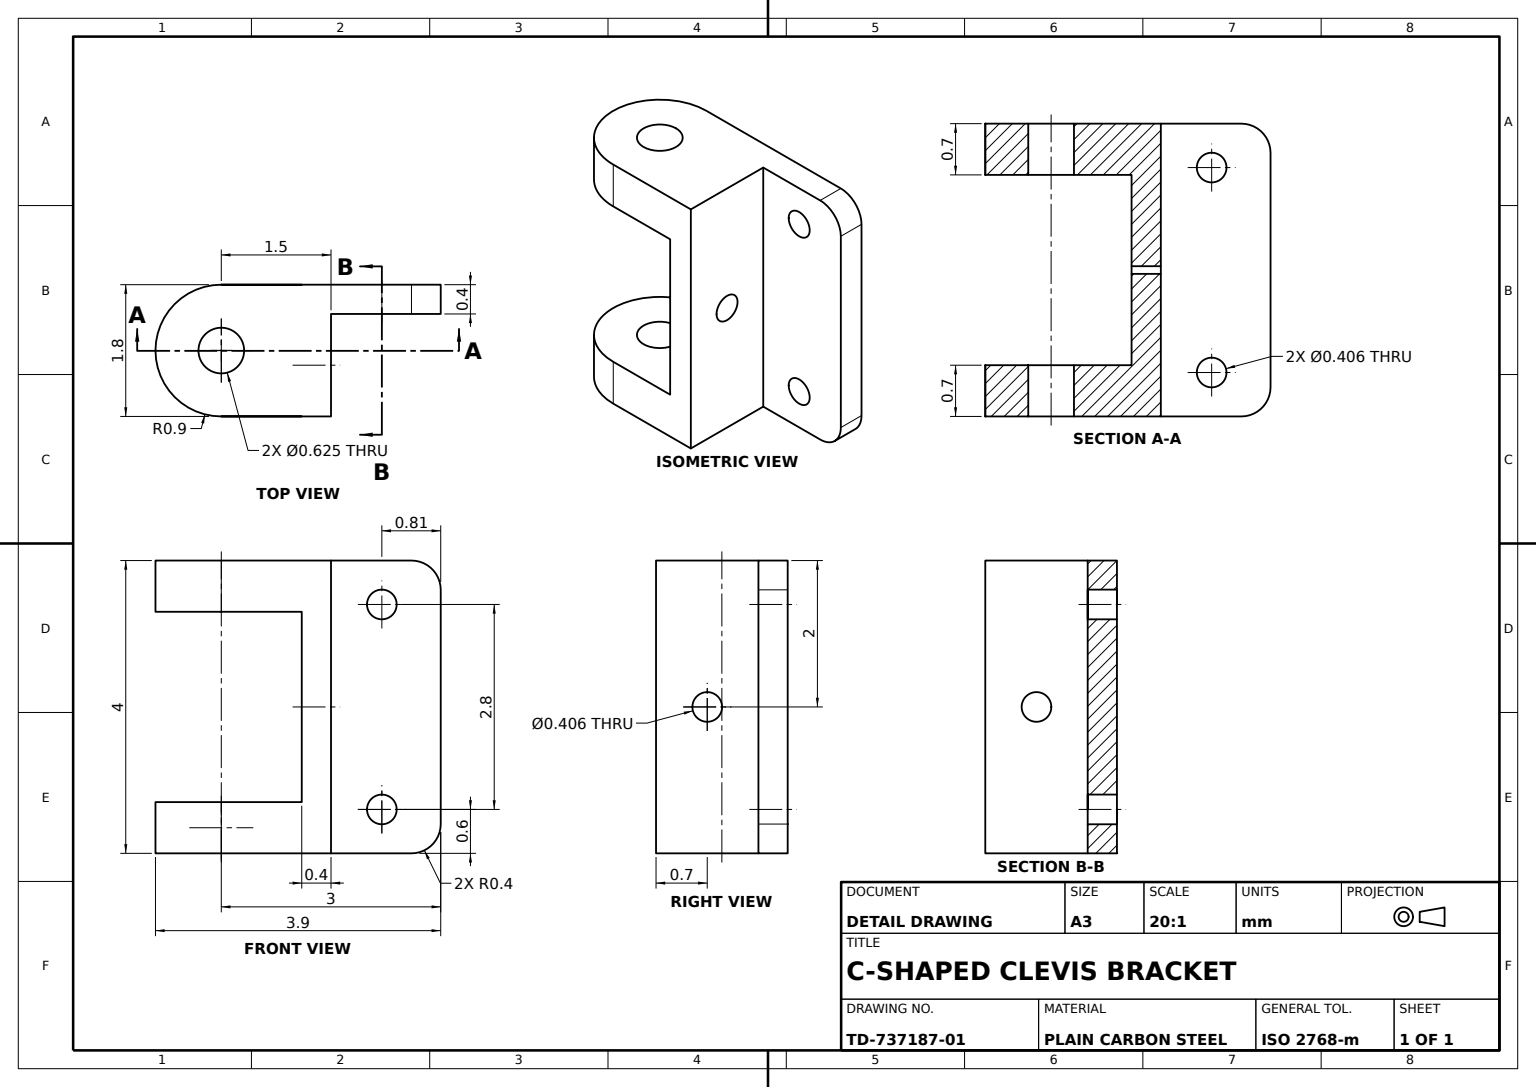
SolidWorks part; units mm, degrees
material "Plain Carbon Steel"
ref_plane "Front Plane" through (0, 0, 0) normal (0, 0, 1) x (1, 0, 0)
ref_plane "Top Plane" through (0, 0, 0) normal (0, 1, 0) x (1, 0, 0)
ref_plane "Right Plane" through (0, 0, 0) normal (1, 0, 0) x (0, 0, -1)
sketch "C-Frame Profile Sketch" plane through (0, 0, 0) normal (0, 0, 1) x (1, 0, 0)
  line L4 (0, 0) -> (2.6, 0)
  line L5 (2.6, -4) -> (0, -4)
  line L6 (0, -4) -> (0, 0)
  line L7 (0, 0) -> (3, 0)
  line L8 (3, -0.4) -> (3, -3.6)
  arc A0 (3, -0.4) -> (2.6, 0) centre (2.6, -0.4) ccw
  arc A1 (3, -3.6) -> (2.6, -4) centre (2.6, -3.6) cw
  point P11 (3, -4)
  dimension "D3" = 0.4
  dimension "D4" = 0.4
  dimension "D1" = 4
  dimension "D2" = 3
extrude "C-Frame Base" add sketch "C-Frame Profile Sketch" along normal blind 0.4 contours A1 L8 A0 L4 L6 L5
sketch "Clevis Gap Sketch" plane through (0, 0, 0) normal (-1, 0, 0) x (0, 0, 1)
  line L0 (0, 0) -> (0.4, 0)
  line L1 (0.4, 0) -> (0.4, -4)
  line L2 (0.4, -4) -> (0, -4)
  line L3 (0, -4) -> (0, 0)
extrude "Clevis Gap Cut" cut sketch "Clevis Gap Sketch" against normal blind 1.5
sketch "Clevis Arm 1 Sketch" plane through (0, 0, 0) normal (0, 1, 0) x (1, 0, 0)
  line L0 (1.5, 0) -> (0, 0)
  line L2 (0, -1.8) -> (1.5, -1.8)
  line L3 (1.5, -1.8) -> (1.5, 0)
  arc A0 (0, 0) -> (0, -1.8) centre (0, -0.9) ccw
  dimension "D1" = 0.9
  dimension "D2" = 1.5
extrude "Clevis Arm 1" add sketch "Clevis Arm 1 Sketch" against normal blind 0.7
sketch "Clevis Arm 2 Sketch" plane through (0, -4, 0) normal (0, -1, 0) x (1, 0, 0)
  line L0 (1.5, 0) -> (0, 0)
  line L2 (0, 1.8) -> (1.5, 1.8)
  line L3 (1.5, 1.8) -> (1.5, 0)
  arc A0 (0, 1.8) -> (0, 0) centre (0, 0.9) ccw
extrude "Clevis Arm 2" add sketch "Clevis Arm 2 Sketch" against normal blind 0.7
sketch "Mounting Flange Sketch" plane through (1.5, 0, 0) normal (-1, 0, 0) x (0, 0, 1)
  line L0 (0, -0.7) -> (1.8, -0.7)
  line L1 (1.8, -0.7) -> (1.8, -3.3)
  line L2 (1.8, -3.3) -> (0, -3.3)
  line L3 (0, -3.3) -> (0, -0.7)
extrude "Mounting Flange" add sketch "Mounting Flange Sketch" along normal blind 0.4
sketch "Back Wall Hole Sketch" plane through (1.5, 0, 0) normal (1, 0, 0) x (0, 0, -1)
  line L0 (-0.4, -4) -> (-1.8, -4) construction
  line L1 (-1.8, -4) -> (-1.8, 0) construction
  circle A0 centre (-1.1, -2) radius 0.203
  dimension "D1" = 0.406
  dimension "D4" = 0.406
  dimension "D2" = 2
  dimension "D3" = 0.7
extrude "Back Wall Hole" cut sketch "Back Wall Hole Sketch" against normal blind 0.4
sketch "Flange Holes Sketch" plane through (0, 0, 0.4) normal (0, 0, 1) x (1, 0, 0)
  line L0 (3, -0.4) -> (3, -3.6) construction
  line L1 (1.5, 0) -> (2.6, 0) construction
  line L2 (2.6, -4) -> (1.5, -4) construction
  circle A0 centre (2.195, -0.6) radius 0.203
  circle A1 centre (2.195, -3.4) radius 0.203
  dimension "D1" = 0.406
  dimension "D2" = 0.406
  dimension "D8" = 0.406
  dimension "D9" = 0.406
  dimension "D3" = 0.805
  dimension "D4" = 0.805
  dimension "D5" = 0.6
  dimension "D6" = 0.6
  dimension "D7" = 2.8
extrude "Flange Holes 2x" cut sketch "Flange Holes Sketch" against normal blind 0.4
sketch "Arm 1 Pin Hole Sketch" plane through (0, 0, 0) normal (0, 1, 0) x (1, 0, 0)
  circle A0 centre (0, -0.9) radius 0.3125
  dimension "D1" = 0.625
  dimension "D2" = 0.625
extrude "Arm 1 Pin Hole" cut sketch "Arm 1 Pin Hole Sketch" against normal blind 0.7
sketch "Arm 2 Pin Hole Sketch" plane through (0, -4, 0) normal (0, -1, 0) x (1, 0, 0)
  circle A0 centre (0, 0.9) radius 0.3125
  dimension "D1" = 0.625
  dimension "D2" = 0.625
extrude "Arm 2 Pin Hole" cut sketch "Arm 2 Pin Hole Sketch" against normal blind 0.7
